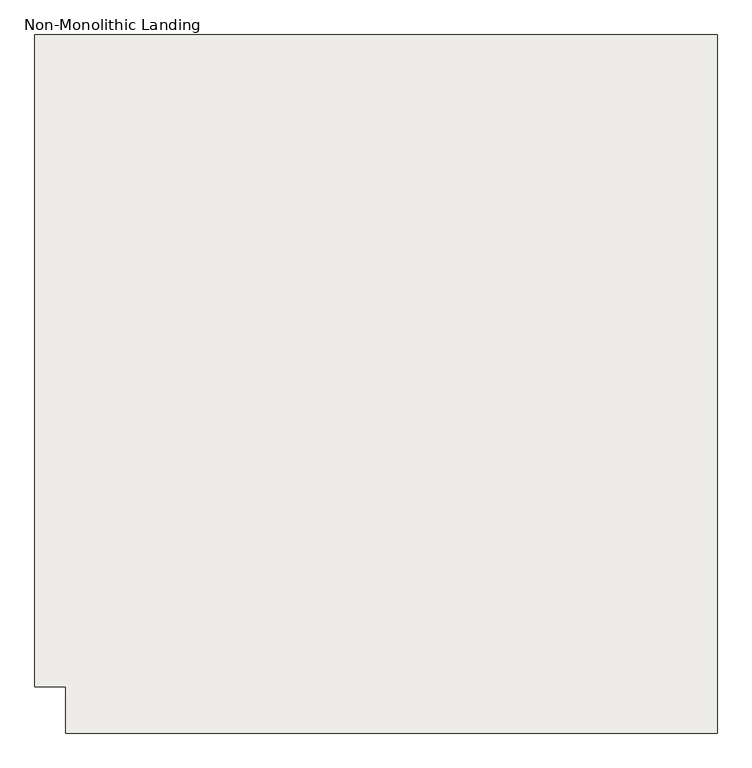
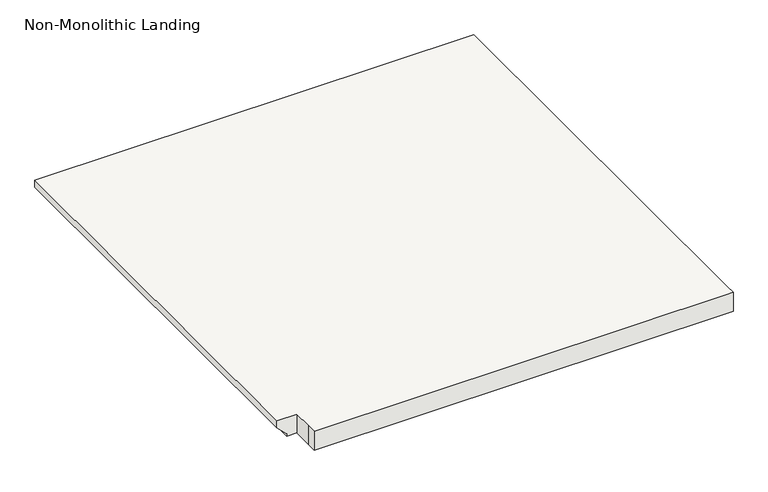
"""IFC4 building model written with IfcOpenShell, lengths in millimetres: slab geometry, Non-Monolithic Landing."""

from ifc_helpers import new_model, si_unit, origin, place, context, project, spatial, faceted_brep, source, transform, mapped, element, save


def non_monolithic_landing_9b4a1add(model_context):
    return source(origin(), model_context, "Body", "Brep", [
        faceted_brep([(2334.73354, -1849.1834702, 4705.35), (2334.73354, -1849.1834702, 4724.4), (2334.73354, -782.3834702, 4724.4), (2334.73354, -782.3834702, 4705.35), (2360.13354, -1849.1834702, 4679.95), (2360.13354, -782.3834702, 4679.95), (2385.53354, -1849.1834702, 4724.4), (2385.53354, -1899.9834702, 4724.4), (2385.53354, -1925.3834702, 4724.4), (3452.33354, -1925.3834702, 4724.4), (3452.33354, -1899.9834702, 4724.4), (3452.33354, -782.3834702, 4724.4), (2360.13354, -1849.1834702, 4673.6), (2360.13354, -782.3834702, 4673.6), (3452.33354, -782.3834702, 4673.6), (3452.33354, -1899.9834702, 4673.6), (3452.33354, -1925.3834702, 4673.6), (2385.53354, -1925.3834702, 4673.6), (2385.53354, -1899.9834702, 4673.6), (2385.53354, -1849.1834702, 4673.6)], [[[0, 1, 2, 3]], [[4, 0, 3, 5]], [[6, 7, 8, 9, 10, 11, 2, 1]], [[12, 13, 14, 15, 16, 17, 18, 19]], [[13, 12, 4, 5]], [[6, 1, 0, 4, 12, 19]], [[7, 6, 19, 18]], [[8, 7, 18, 17]], [[9, 8, 17, 16]], [[10, 9, 16, 15]], [[11, 10, 15, 14]], [[2, 11, 14, 13, 5, 3]]]),
    ])


if __name__ == "__main__":
    model = new_model("IFC4")
    model_context = context("Model", 3, world=origin())
    ifc_project = project(units=[si_unit("LENGTHUNIT", "METRE", prefix="MILLI")], contexts=[model_context])
    site = spatial("IfcSite", under=ifc_project)
    building = spatial("IfcBuilding", under=site)
    placement = place(None, origin())
    non_monolithic_landing_shape = non_monolithic_landing_9b4a1add(model_context)
    element("IfcSlab", 1, ObjectType="Non-Monolithic Landing", at=placement, inside=building, context=model_context, shape_type="MappedRepresentation", body=[
        mapped(non_monolithic_landing_shape, transform((0.0, 0.0, 0.0), x_axis=(1.0, 0.0, 0.0), y_axis=(0.0, 1.0, 0.0), z_axis=(0.0, 0.0, 1.0))),
    ])
    save(model, "model.ifc")
